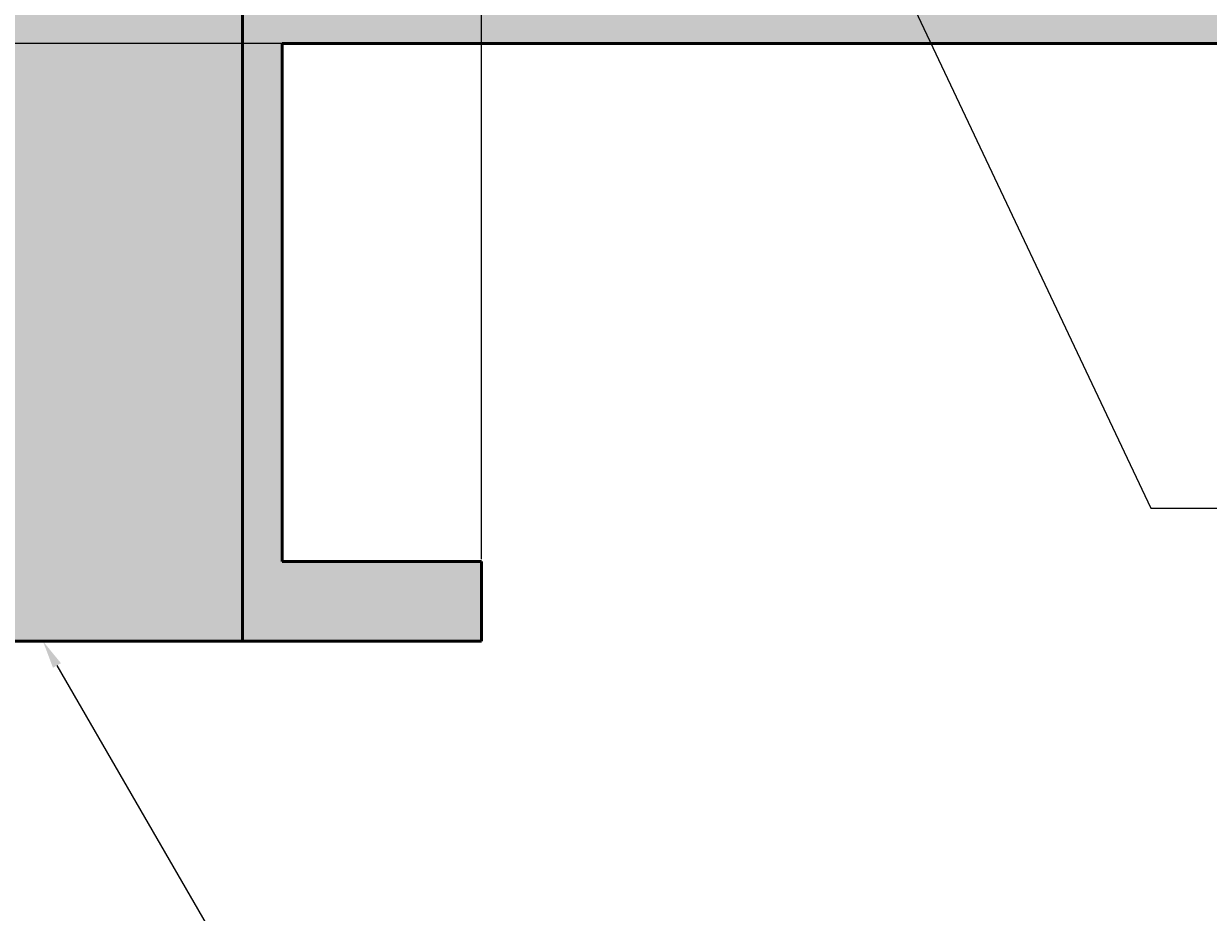
# Model space of a CAD drawing. Units: inches. Extents: x -12 to 334, y -10 to 186.
# Tile 49 of 77: x 227 to 257, y 24 to 46. Entities that reach past the tile are written whole.
import ezdxf
from ezdxf import colors
from ezdxf.entities.mleader import LeaderData, LeaderLine
from ezdxf.math import Vec2, Vec3

# ---------------------------------------------------------------- set-up
doc = ezdxf.new("R2010")
doc.units = ezdxf.units.IN
doc.header["$MEASUREMENT"] = 0
for name, color, linetype, lineweight in [('M-ANNO-TEXT', 3, 'Continuous', 25), ('M-DIMS', 2, 'Continuous', 18), ('M-EQPM', 7, 'Continuous', 50), ('M-EQPM-PATT', 8, 'Continuous', 18)]:
    doc.layers.add(name, color=color, linetype=linetype, lineweight=lineweight)
doc.styles.get("Standard").update_dxf_attribs({"font": 'arial.ttf'})
doc.dimstyles.get("Standard").update_dxf_attribs({"dimtxt": 0.18, "dimasz": 0.18, "dimexe": 0.18, "dimexo": 0.0625, "dimgap": 0.09, "dimtad": 0, "dimtih": 1, "dimtoh": 1, "dimdec": 4, "dimzin": 0, "dimdsep": 46, "dimtxsty": 'Standard', "dimcen": 0.09, "dimadec": 0, "dimazin": 0, "dimtfac": 1, "dimtdec": 4, "dimtofl": 0, "dimtmove": 0, "dimatfit": 3, "dimfxl": 1, "dimtolj": 1, "dimtzin": 0, "dimarcsym": 0})

# ---------------------------------------------------------------- blocks, each defined once
blk = doc.blocks.new('*D1')
at = {"layer": 'Defpoints', "color": 0, "transparency": 16777216}
for p in [(281.426, 91.899), (3.376, 80.692), (281.426, 14.304)]:
    blk.add_point(p, dxfattribs=at)
at = {"layer": 'M-DIMS', "color": 0, "lineweight": -2, "transparency": 16777216}
for p, q in [((281.426, 91.836), (281.426, 14.124)), ((3.376, 80.629), (3.376, 14.124)), ((3.556, 14.304), (141.935, 14.304)), ((281.246, 14.304), (142.867, 14.304))]:
    blk.add_line(p, q, dxfattribs=at)
at = {"layer": 'M-DIMS', "color": 0, "transparency": 16777216}
for points in [[(3.556, 14.334), (3.556, 14.274), (3.376, 14.304)], [(281.246, 14.334), (281.246, 14.274), (281.426, 14.304)]]:
    blk.add_solid(points, dxfattribs=at)
at = {"layer": 'M-DIMS', "color": 0, "transparency": 16777216, "insert": (142.401, 14.304), "char_height": 0.18, "attachment_point": 5}
blk.add_mtext('\\A1;278.05', dxfattribs=at)
blk = doc.blocks.new('*D27')
at = {"layer": 'Defpoints', "color": 0, "transparency": 16777216}
for p in [(238.576, 169.385), (216.576, 32.854), (238.576, 32.854)]:
    blk.add_point(p, dxfattribs=at)
at = {"layer": 'M-DIMS', "color": 0, "lineweight": -2, "transparency": 16777216}
for p, q in [((216.576, 32.917), (216.576, 169.565)), ((216.756, 169.385), (227.357, 169.385)), ((238.396, 169.385), (227.796, 169.385)), ((238.576, 32.917), (238.576, 169.565))]:
    blk.add_line(p, q, dxfattribs=at)
at = {"layer": 'M-DIMS', "color": 0, "transparency": 16777216}
for points in [[(216.756, 169.415), (216.756, 169.355), (216.576, 169.385)], [(238.396, 169.415), (238.396, 169.355), (238.576, 169.385)]]:
    blk.add_solid(points, dxfattribs=at)
at = {"layer": 'M-DIMS', "color": 0, "transparency": 16777216, "insert": (227.576, 169.385), "char_height": 0.18, "attachment_point": 5}
blk.add_mtext('\\A1;22', dxfattribs=at)
blk = doc.blocks.new('*D28')
at = {"layer": 'Defpoints', "color": 0, "transparency": 16777216}
for p in [(232.576, 169.385), (222.576, 30.854), (232.576, 30.854)]:
    blk.add_point(p, dxfattribs=at)
at = {"layer": 'M-DIMS', "color": 0, "lineweight": -2, "transparency": 16777216}
for p, q in [((222.576, 30.917), (222.576, 169.565)), ((222.756, 169.385), (227.366, 169.385)), ((232.396, 169.385), (227.786, 169.385)), ((232.576, 30.917), (232.576, 169.565))]:
    blk.add_line(p, q, dxfattribs=at)
at = {"layer": 'M-DIMS', "color": 0, "transparency": 16777216}
for points in [[(222.756, 169.415), (222.756, 169.355), (222.576, 169.385)], [(232.396, 169.415), (232.396, 169.355), (232.576, 169.385)]]:
    blk.add_solid(points, dxfattribs=at)
at = {"layer": 'M-DIMS', "color": 0, "transparency": 16777216, "insert": (227.576, 169.385), "char_height": 0.18, "attachment_point": 5}
blk.add_mtext('\\A1;10', dxfattribs=at)
blk = doc.blocks.new('*D39')
at = {"layer": 'Defpoints', "color": 0, "transparency": 16777216}
for p in [(279.726, 80.692), (-11.174, 45.854), (269.381, 45.854)]:
    blk.add_point(p, dxfattribs=at)
at = {"layer": 'M-DIMS', "color": 0, "lineweight": -2, "transparency": 16777216}
for p, q in [((279.664, 80.692), (-11.354, 80.692)), ((-11.174, 80.512), (-11.174, 63.455)), ((-11.174, 46.034), (-11.174, 63.091)), ((269.318, 45.854), (-11.354, 45.854))]:
    blk.add_line(p, q, dxfattribs=at)
at = {"layer": 'M-DIMS', "color": 0, "transparency": 16777216}
for points in [[(-11.204, 80.512), (-11.144, 80.512), (-11.174, 80.692)], [(-11.204, 46.034), (-11.144, 46.034), (-11.174, 45.854)]]:
    blk.add_solid(points, dxfattribs=at)
at = {"layer": 'M-DIMS', "color": 0, "transparency": 16777216, "insert": (-11.174, 63.273), "char_height": 0.18, "attachment_point": 5}
blk.add_mtext('\\A1;34.84', dxfattribs=at)

msp = doc.modelspace()

# ---------------------------------------------------------------- hatches: boundary and pattern name
at = {"layer": 'M-EQPM-PATT'}
h = msp.add_hatch(color=256, dxfattribs=at)
h.set_gradient(color1=(99, 100, 102), color2=(99, 100, 102), tint=1)
h.paths.add_polyline_path([(126.9567, 136.8871), (179.7818, 136.8871), (180.0106, 137.8871), (126.3793, 137.8871), (106.1771, 102.8958), (86.8879, 102.8958), (86.8879, 109.0583), (84.7229, 109.0583), (84.7229, 100.8958), (106.1771, 100.8958)])
h.paths.add_polyline_path([(196.3421, 152.8345), (195.3421, 152.8345), (195.3421, 137.8871), (180.0106, 137.8871), (179.7818, 136.8871), (196.3421, 136.8871)])
h.paths.add_polyline_path([(215.0166, 152.8345), (214.0166, 152.8345), (214.0166, 136.9435), (268.3808, 136.9435, -0.2673785), (268.3808, 46.8541), (249.3759, 46.8541), (249.8485, 45.8541), (269.3808, 45.8541, 0.2615891), (269.3808, 137.9435), (215.0166, 137.9435)])
h = msp.add_hatch(color=256, dxfattribs=at)
h.set_gradient(color1=(99, 100, 102), color2=(99, 100, 102), tint=1)
h.paths.add_polyline_path([(4.3766, 80.754, -0.4132606), (23.5807, 99.8958), (37.1002, 99.8958), (37.1002, 127.7078), (32.1002, 127.7078), (32.1002, 125.2078), (36.1002, 125.2078), (36.1002, 100.8958), (23.5807, 100.8958, 1), (23.5807, 60.4872), (36.1002, 60.4872), (36.1002, 36.1752), (32.1002, 36.1752), (32.1002, 33.6752), (37.1002, 33.6752), (37.1002, 61.4872), (23.5807, 61.4872, -0.384914), (4.4744, 78.754), (72.9244, 78.754), (72.9244, 69.6117), (75.9244, 69.6117), (75.9244, 89.8963), (72.9244, 89.8963), (72.9244, 80.754)])
h.paths.add_polyline_path([(54.1002, 125.2078), (58.1002, 125.2078), (58.1002, 127.7078), (53.1002, 127.7078), (53.1002, 99.8958), (64.5, 99.8958), (64.5, 109.0583), (63.5, 109.0583), (63.5, 100.8958), (54.1002, 100.8958)], flags=17)
h.paths.add_polyline_path([(53.1002, 33.6752), (58.1002, 33.6752), (58.1002, 36.1752), (54.1002, 36.1752), (54.1002, 60.4872), (64.2068, 60.4872), (64.2068, 49.4497), (87.8879, 49.4497), (87.8879, 55.3205), (104.8919, 55.3205), (104.8919, 30.8541), (99.8919, 30.8541), (99.8919, 28.8541), (105.8919, 28.8541), (105.8919, 56.3205), (87.8879, 56.3205), (87.8879, 63.6117), (86.8879, 63.6117), (86.8879, 50.4497), (65.0061, 50.4497), (65.0061, 63.6117), (64.5, 63.6117), (64.5, 61.4872), (53.1002, 61.4872)])
h.paths.add_polyline_path([(121.8919, 28.8541), (121.8919, 30.8541), (116.8919, 30.8541), (116.8919, 45.8541), (209.6965, 45.8541), (209.9204, 46.8541), (115.8919, 46.8541), (115.8919, 28.8541)])
h.paths.add_polyline_path([(221.5761, 32.8541), (216.5761, 32.8541), (216.5761, 30.8541), (222.5761, 30.8541), (222.5761, 46.8541), (209.9204, 46.8541), (209.6965, 45.8541), (221.5761, 45.8541)])
h.paths.add_polyline_path([(233.5761, 45.8541), (249.8485, 45.8541), (249.3759, 46.8541), (232.5761, 46.8541), (232.5761, 30.8541), (238.5761, 30.8541), (238.5761, 32.8541), (233.5761, 32.8541)])
h = msp.add_hatch(color=256, dxfattribs=at)
h.set_gradient(color1=(94, 103, 175), color2=(94, 103, 175), tint=1)
h.paths.add_polyline_path([(129.093, 89.8963), (86.8879, 89.8963), (86.8879, 69.6117), (129.093, 69.6117)], flags=17)
h.paths.add_polyline_path([(170.9079, 89.8963), (130.8573, 89.8963), (130.8573, 69.6117), (170.9079, 69.6117)], flags=17)
h.paths.add_polyline_path([(216.4278, 89.8963), (172.6722, 89.8963), (172.6722, 69.6117), (216.4278, 69.6117)], flags=17)
h.paths.add_polyline_path([(245.9354, 82.6969), (247.9354, 82.6969), (247.9354, 46.8541), (268.3808, 46.8541, 0.0998398), (279.7263, 80.6915), (251.9801, 80.6915, 0.4142136), (231.7758, 100.8958), (84.7229, 100.8958), (84.7229, 109.0583), (83.7229, 109.0583), (83.7229, 95.8963), (129.093, 95.8963), (129.093, 98.1081), (130.8573, 98.1081), (130.8573, 95.8963), (170.9079, 95.8963), (170.9079, 98.1081), (172.6722, 98.1081), (172.6722, 95.8963), (216.4278, 95.8963), (216.4278, 98.1081), (218.1922, 98.1081), (218.1922, 95.8963), (226.6083, 95.8963, -1), (226.6083, 63.6117), (218.1922, 63.6117), (218.1922, 61.1045), (216.4278, 61.1045), (216.4278, 63.6117), (172.6722, 63.6117), (172.6722, 61.1045), (170.9079, 61.1045), (170.9079, 63.6117), (130.8573, 63.6117), (130.8573, 61.1045), (129.093, 61.1045), (129.093, 63.6117), (87.8879, 63.6117), (87.8879, 56.3205), (105.8919, 56.3205), (105.8919, 28.8541), (115.8919, 28.8541), (115.8919, 46.8541), (222.5761, 46.8541), (222.5761, 30.8541), (232.5761, 30.8541), (232.5761, 46.8541), (245.9354, 46.8541)])
h.paths.add_polyline_path([(86.8879, 89.8963), (75.9244, 89.8963), (75.9244, 69.6117), (86.8879, 69.6117)])
h.paths.add_polyline_path([(83.7229, 109.0583), (75.9244, 109.0583), (75.9244, 95.8963), (83.7229, 95.8963)])
h.paths.add_polyline_path([(226.6083, 89.8963), (218.1922, 89.8963), (218.1922, 69.6117), (226.6083, 69.6117, 1)], flags=17)
h = msp.add_hatch(color=256, dxfattribs=at)
h.set_gradient(color1=(0, 0, 255), color2=(0, 0, 255), tint=1)
h.paths.add_polyline_path([(84.7229, 100.8958), (84.7229, 109.0583), (83.7229, 109.0583), (83.7229, 95.8963), (129.093, 95.8963), (129.093, 98.1081), (130.8573, 98.1081), (130.8573, 95.8963), (170.9079, 95.8963), (170.9079, 98.1081), (172.6722, 98.1081), (172.6722, 95.8963), (216.4278, 95.8963), (216.4278, 98.1081), (218.1922, 98.1081), (218.1922, 95.8963), (226.6083, 95.8963, -1), (226.6083, 63.6117), (218.1922, 63.6117), (218.1922, 61.1045), (216.4278, 61.1045), (216.4278, 63.6117), (172.6722, 63.6117), (172.6722, 61.1045), (170.9079, 61.1045), (170.9079, 63.6117), (130.8573, 63.6117), (130.8573, 61.1045), (129.093, 61.1045), (129.093, 63.6117), (87.8879, 63.6117), (87.8879, 56.3205), (105.8919, 56.3205), (105.8919, 28.8541), (115.8919, 28.8541), (115.8919, 46.8541), (222.5761, 46.8541), (222.5761, 30.8541), (232.5761, 30.8541), (232.5761, 46.8541), (245.9354, 46.8541), (245.9354, 82.6969), (247.9354, 82.6969), (247.9354, 46.8541), (268.3808, 46.8541, 0.0998398), (279.7263, 80.6915), (251.9801, 80.6915, 0.4142136), (231.7758, 100.8958)])

# ---------------------------------------------------------------- linework, layer by layer
at = {"layer": 'M-EQPM'}
for p, q in [((232.5761, 46.8541), (232.5761, 30.8541)), ((269.3808, 45.8541), (233.5761, 45.8541)), ((233.5761, 45.8541), (233.5761, 32.8541)), ((233.5761, 32.8541), (238.5761, 32.8541)), ((238.5761, 32.8541), (238.5761, 30.8541)), ((216.5761, 30.8541), (238.5761, 30.8541)), ((233.5761, 30.8541), (221.5761, 30.8541))]:
    msp.add_line(p, q, dxfattribs=at)

# ---------------------------------------------------------------- dimensions: what is measured, and where the dimension line sits
at = {"layer": 'M-DIMS'}
for base, p1, p2, override, picture, middle in [((238.5761, 169.3845), (216.5761, 32.8541), (238.5761, 32.8541), {"dimdec": 0, "dimlfac": 1, "dimrnd": 0, "dimzin": 0, "dimdsep": 46, "dimlunit": 2}, '*D27', (227.5761, 169.3845)), ((232.5761, 169.3845), (222.5761, 30.8541), (232.5761, 30.8541), {"dimdec": 0, "dimlfac": 1, "dimrnd": 0, "dimzin": 0, "dimdsep": 46, "dimlunit": 2}, '*D28', (227.5761, 169.3845)), ((281.4256, 14.3041), (3.3765, 80.6915), (281.4256, 91.8988), {"dimdec": 2, "dimlfac": 1, "dimrnd": 0, "dimzin": 0, "dimdsep": 46, "dimlunit": 2}, '*D1', (142.401, 14.3041))]:
    dim = msp.add_linear_dim(base=base, p1=p1, p2=p2, dimstyle='Standard', override=override, dxfattribs=at)
    dim.commit()
    dim.dimension.update_dxf_attribs({"geometry": picture, "text_midpoint": middle})
dim = msp.add_linear_dim(base=(-11.1736, 45.8541), p1=(279.7263, 80.6915), p2=(269.3808, 45.8541), angle=90, dimstyle='Standard', override={"dimdec": 2, "dimlfac": 1, "dimrnd": 0, "dimzin": 0, "dimdsep": 46, "dimlunit": 2}, dxfattribs=at)
dim.commit()
dim.dimension.update_dxf_attribs({"geometry": '*D39', "text_midpoint": (-11.1735, 63.2728)})

# ---------------------------------------------------------------- leaders
at = {"layer": 'M-ANNO-TEXT'}
ml = msp.add_multileader_mtext('Standard', dxfattribs=at)
ml.set_content('^I^IWeir', color=256)
ml.set_leader_properties()
ml.build(insert=Vec2(0, 0))
ml.multileader.update_dxf_attribs({"dogleg_length": 0.36, "arrow_head_size": 0.7})
ctx = ml.context
ctx.base_point, ctx.arrow_head_size, ctx.landing_gap_size, ctx.plane_origin = Vec3(257.1525, 34.1955), 0.7, 0.09, Vec3(247.9354, 49.9015)
notes = []
notes.append((ctx, [(0, (1, 1, 0), (255.3593, 34.1955), (1, 0), 1.7932, [(0, [(247.9354, 49.9015)], 0, [])])]))
ctx.mtext.insert, ctx.mtext.flow_direction = Vec3(257.2425, 36.2283), 5
ml = msp.add_multileader_mtext('Standard', dxfattribs=at)
ml.set_content('Bottom product', color=256)
ml.set_leader_properties()
ml.build(insert=Vec2(0, 0))
ml.multileader.update_dxf_attribs({"dogleg_length": 0.36, "arrow_head_size": 0.7})
ctx = ml.context
ctx.base_point, ctx.arrow_head_size, ctx.landing_gap_size, ctx.plane_origin = Vec3(237.0261, 20.0676), 0.7, 0.09, Vec3(227.5761, 30.8541)
notes.append((ctx, [(0, (1, 1, 0), (233.8037, 20.0676), (1, 0), 3.2224, [(0, [(227.5761, 30.8541)], 0, [])])]))
ctx.mtext.insert, ctx.mtext.flow_direction = Vec3(237.1161, 22.6228), 5
for ctx, leaders in notes:
    for number, flags, end, landing, length, lines in leaders:
        leader = LeaderData()
        leader.index, (leader.has_last_leader_line, leader.has_dogleg_vector, leader.attachment_direction) = number, flags
        leader.last_leader_point, leader.dogleg_vector, leader.dogleg_length = Vec3(end), Vec3(landing), length
        for number, points, colour, breaks in lines:
            line = LeaderLine()
            line.index, line.vertices, line.color, line.breaks = number, Vec3.list(points), colors.encode_raw_color(colour), breaks
            leader.lines.append(line)
        ctx.leaders.append(leader)

doc.saveas('drawing.dxf')
